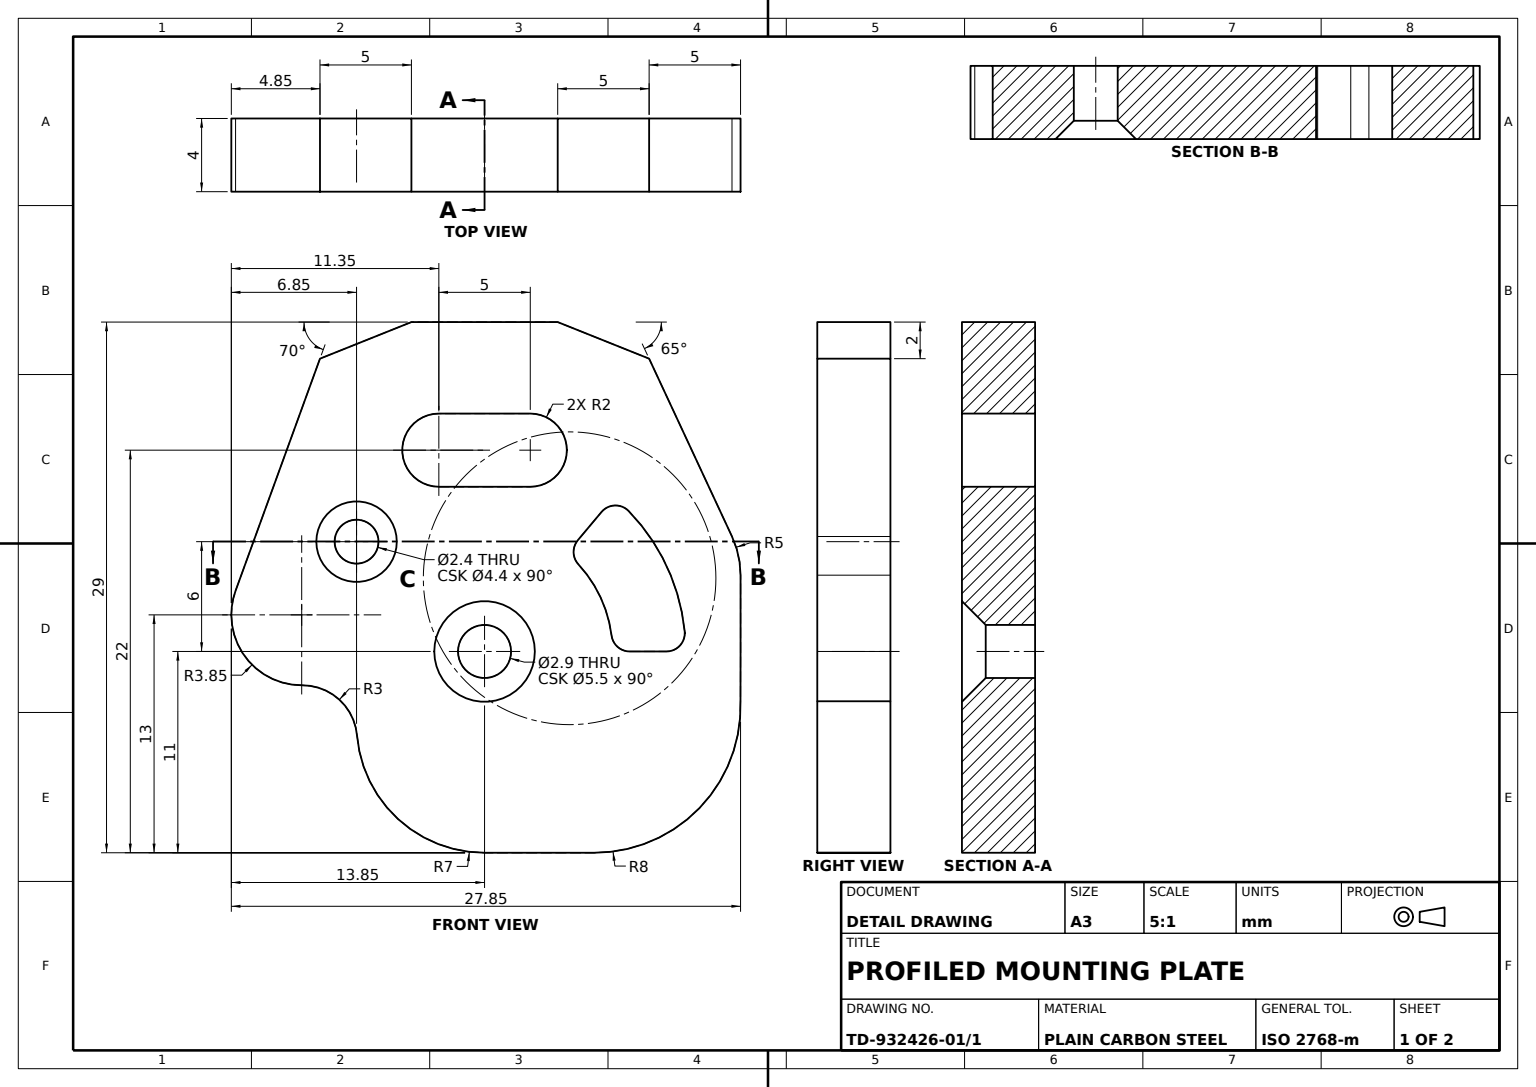
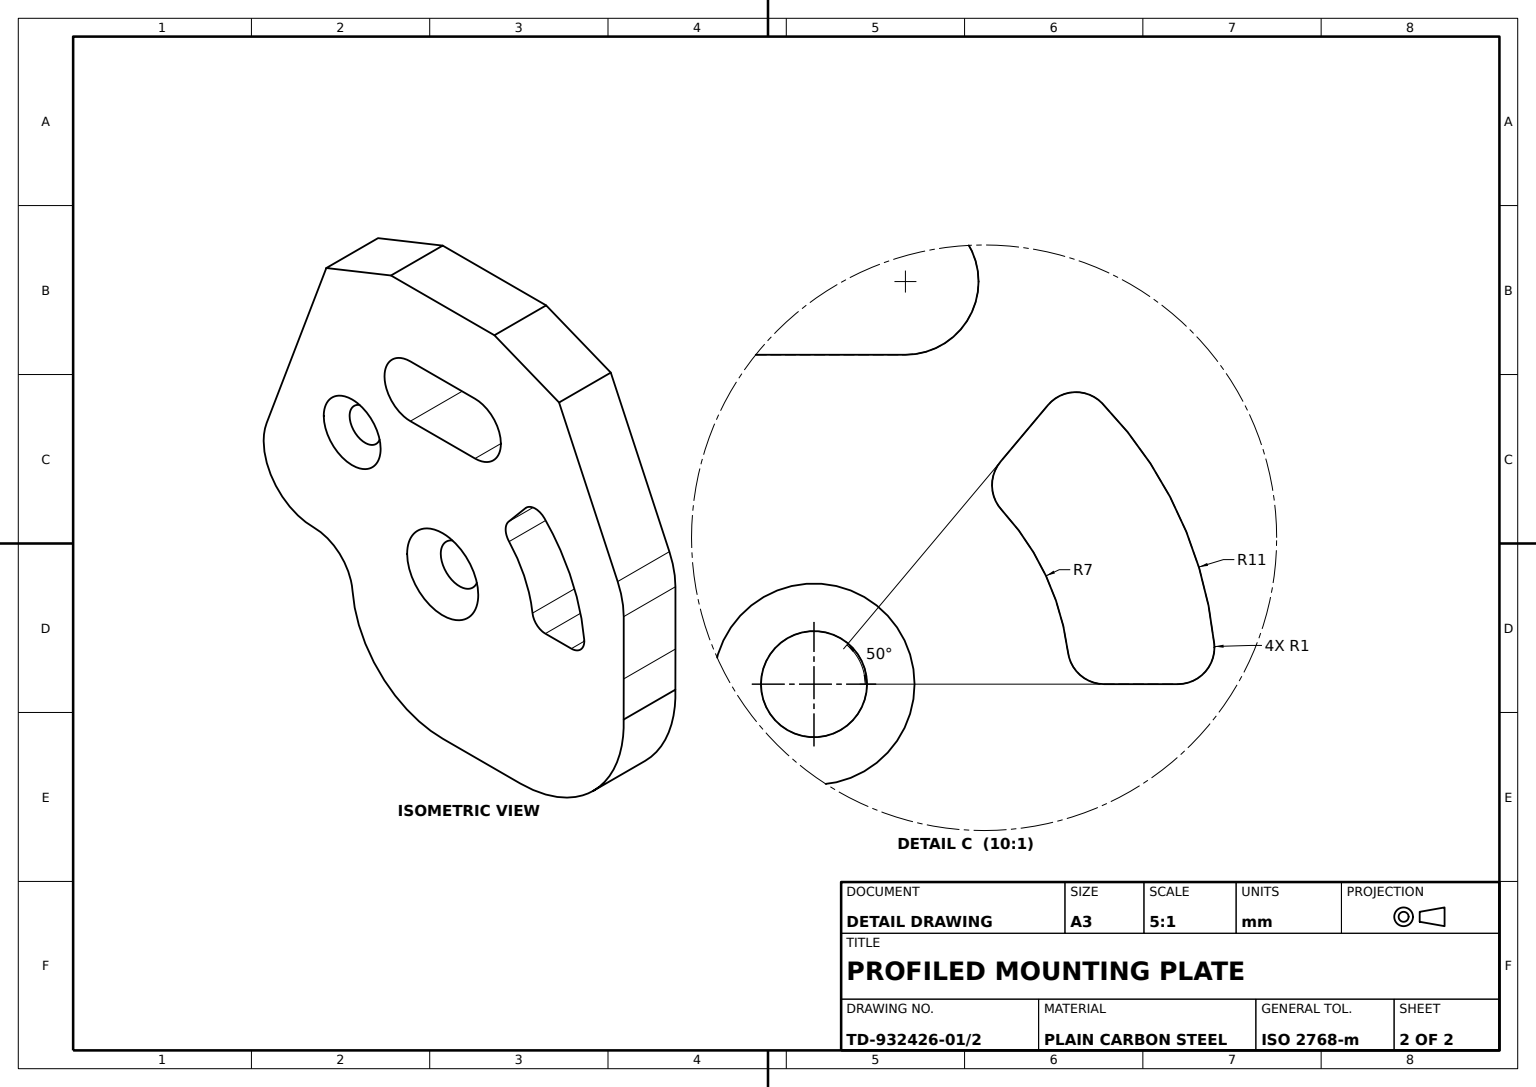
from build123d import *

# Parameters (mm, degrees)
CAM_PLATE_4MM_DEPTH       = 4
SLOTS_CUT_DEPTH           = 4
CSK_HOLE_M2_5_D           = 2.9
CSK_HOLE_M2_5_DEPTH       = 29
CSK_HOLE_M2_5_CSINK_D     = 5.5
CSK_HOLE_M2_5_CSINK_ANGLE = 90
CSK_HOLE_M2_5_TIP         = 0.871247898
CSK_HOLE_M2_D             = 2.4
CSK_HOLE_M2_DEPTH         = 29
CSK_HOLE_M2_CSINK_D       = 4.4
CSK_HOLE_M2_CSINK_ANGLE   = 90
CSK_HOLE_M2_TIP           = 0.721032743


with BuildPart() as part:
    # Cam Plate Profile Sketch → Cam Plate 4mm (new body)
    with BuildSketch(Plane.XY):
        with BuildLine():
            Line((4, 4.474241718), (-4, 4.474241718))
            Line((-4, 4.474241718), (-9, 2.474241718))
            Line((-9, 2.474241718), (-13.616491046, -10.209463189))
            ThreePointArc((-13.616491046, -10.209463189), (-13.146761684, -13.741504469), (-9.979750738, -15.374294397))
            ThreePointArc((-9.979750738, -15.374294397), (-7.940438794, -16.159442387), (-6.974754793, -18.11972425))
            ThreePointArc((-6.974754793, -18.11972425), (-4.735094414, -22.681229249), (0, -24.525758282))
            Line((0, -24.525758282), (6, -24.525758282))
            ThreePointArc((6, -24.525758282), (11.754495804, -22.083255744), (13.995148957, -16.247202791))
            Line((13.995148957, -16.247202791), (14, -13.525758282))
            Line((14, -13.525758282), (14, -9.356766198))
            ThreePointArc((14, -9.356766198), (13.881480036, -8.274568128), (13.531538935, -7.243674889))
            Line((13.531538935, -7.243674889), (9, 2.474241718))
            Line((9, 2.474241718), (4, 4.474241718))
        make_face()
    extrude(amount=CAM_PLATE_4MM_DEPTH)

    # Slot Profiles Sketch → Slots Cut (cut)
    with BuildSketch(Plane.XY.offset(4)):
        with BuildLine():
            Line((-2.5, -0.525758282), (2.5, -0.525758282))
            ThreePointArc((2.5, -0.525758282), (4.5, -2.525758282), (2.5, -4.525758282))
            Line((2.5, -4.525758282), (-2.5, -4.525758282))
            ThreePointArc((-2.5, -4.525758282), (-4.5, -2.525758282), (-2.5, -0.525758282))
        make_face()
        with BuildLine():
            Line((5.101968483, -7.445469013), (6.395655964, -5.90371231))
            ThreePointArc((6.395655964, -5.90371231), (7.124526222, -5.547191119), (7.877870447, -5.848574084))
            ThreePointArc((7.877870447, -5.848574084), (9.969385657, -8.876957403), (10.944861808, -12.425758282))
            ThreePointArc((10.944861808, -12.425758282), (10.69149422, -13.196578675), (9.949874371, -13.525758282))
            Line((9.949874371, -13.525758282), (7.937253933, -13.525758282))
            ThreePointArc((7.937253933, -13.525758282), (7.275816105, -13.275758282), (6.945097192, -12.650758282))
            ThreePointArc((6.945097192, -12.650758282), (6.344154509, -10.56743045), (5.134511311, -8.76794433))
            ThreePointArc((5.134511311, -8.76794433), (4.868315554, -8.112856688), (5.101968483, -7.445469013))
        make_face()
    extrude(amount=-SLOTS_CUT_DEPTH, mode=Mode.SUBTRACT)

    # CSK Hole M2.5
    with Locations(Plane(origin=(0, -13.525758282, 4), x_dir=(1, 0, 0), z_dir=(0, 0, 1))):
        with Locations((0, 0)):
            CounterSinkHole(CSK_HOLE_M2_5_D / 2, CSK_HOLE_M2_5_CSINK_D / 2, depth=CSK_HOLE_M2_5_DEPTH, counter_sink_angle=CSK_HOLE_M2_5_CSINK_ANGLE)
            with Locations((0, 0, -(CSK_HOLE_M2_5_DEPTH + CSK_HOLE_M2_5_TIP / 2))):  # 118° drill point
                Cone(0, CSK_HOLE_M2_5_D / 2, CSK_HOLE_M2_5_TIP, mode=Mode.SUBTRACT)

    # CSK Hole M2
    with Locations(Plane(origin=(-7, -7.525758282, 4), x_dir=(1, 0, 0), z_dir=(0, 0, 1))):
        with Locations((0, 0)):
            CounterSinkHole(CSK_HOLE_M2_D / 2, CSK_HOLE_M2_CSINK_D / 2, depth=CSK_HOLE_M2_DEPTH, counter_sink_angle=CSK_HOLE_M2_CSINK_ANGLE)
            with Locations((0, 0, -(CSK_HOLE_M2_DEPTH + CSK_HOLE_M2_TIP / 2))):  # 118° drill point
                Cone(0, CSK_HOLE_M2_D / 2, CSK_HOLE_M2_TIP, mode=Mode.SUBTRACT)


solid = part.part
